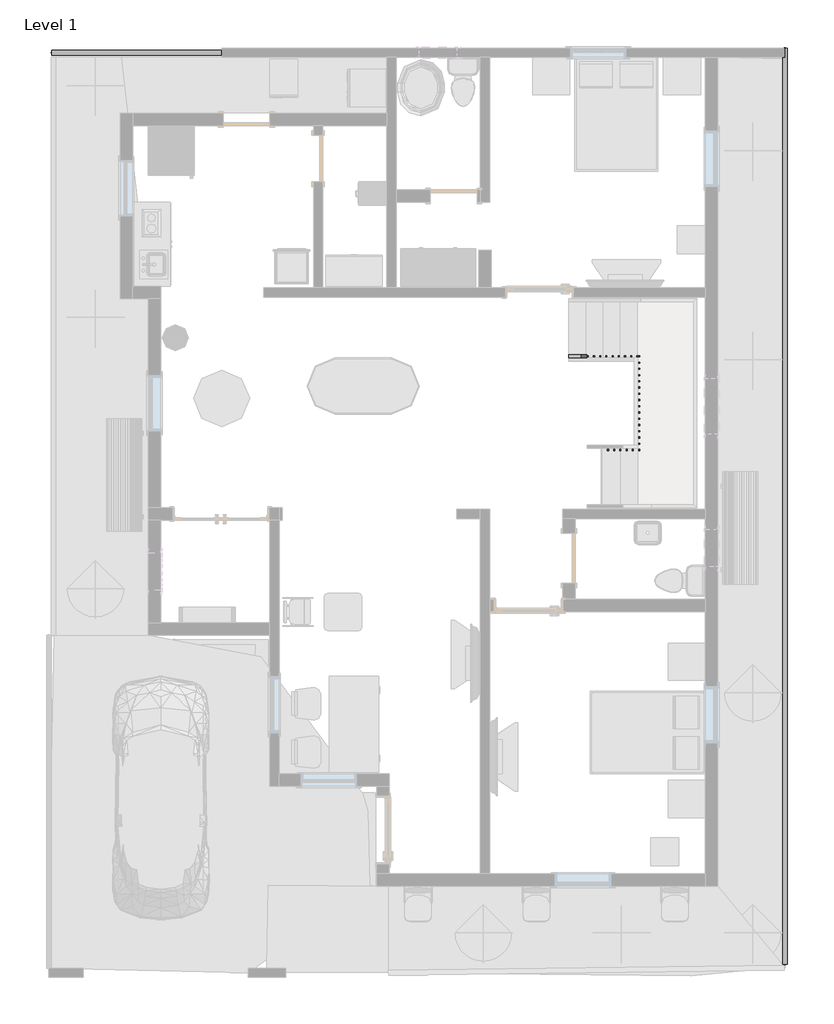
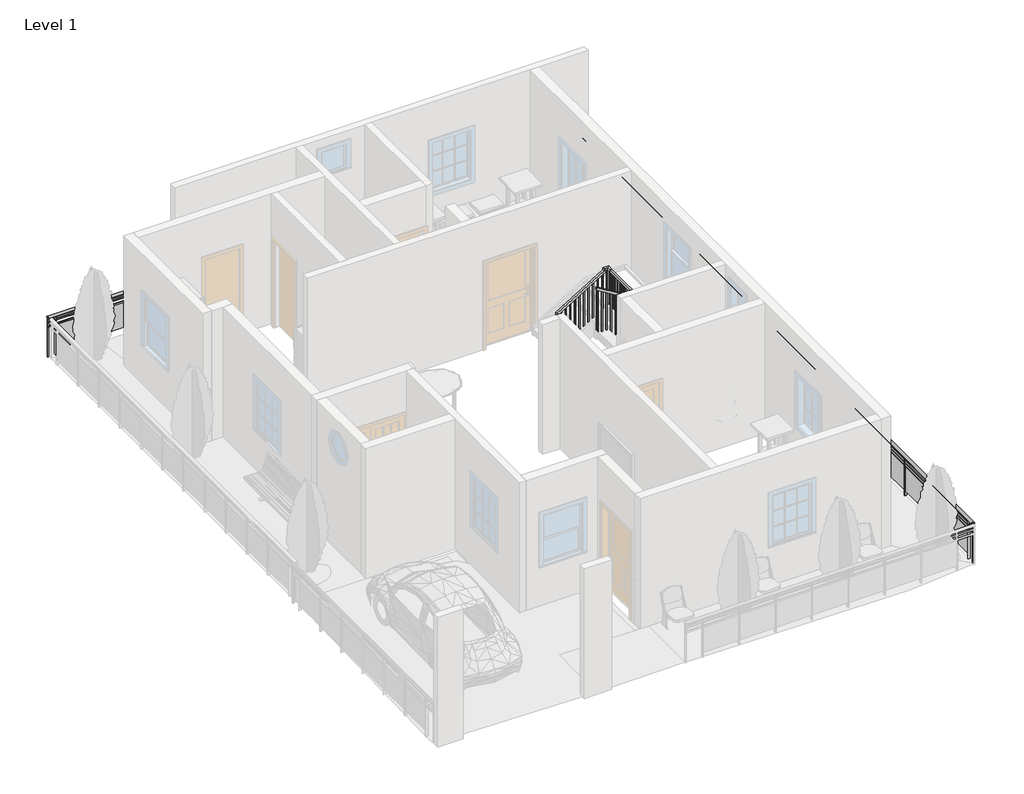
# One storey, part 3 of 4: 3 railings.
"""IFC4 building model written with IfcOpenShell, lengths in millimetres."""

from ifc_helpers import new_model, si_unit, point, frame, origin, origin_with_axes, place, context, project, spatial, polyline, ellipse_curve, trimmed, outline, extrude, faceted_brep, element, save
from ifc_brep_helpers import plane_surface, extruded_surface, advanced_brep

model = new_model("IFC4")

# Units and contexts
model_context = context("Model", 3, world=origin())
ifc_project = project(units=[si_unit("LENGTHUNIT", "METRE", prefix="MILLI")], contexts=[model_context])

# Site, building, storey
site = spatial("IfcSite", under=ifc_project)
building = spatial("IfcBuilding", under=site)
storey = spatial("IfcBuildingStorey", under=building, Name="Level 1", Elevation=0.0)

# Railings
placement = place(None, origin())
element("IfcRailing", 1, ObjectType="Glass Panel - Bottom Fill", at=placement, inside=storey, context=model_context, shape_type="SolidModel", body=[
    advanced_brep(
    [(-5161.8434793, 15525.6426639, 914.4), (-5238.0434793, 15525.6426639, 914.4), (-5161.8434793, 590.4426639, 914.4), (-5238.0434793, 590.4426639, 914.4)],
    [
        (0, 1, ellipse_curve(frame((-5199.9434793, 15525.6426639, 914.4), z_axis=(0.0, 1.0, 0.0), x_axis=(-1.0, 0.0, 0.0)), 38.1, 28.575)),
        (1, 0, ellipse_curve(frame((-5199.9434793, 15525.6426639, 914.4), z_axis=(0.0, 1.0, 0.0), x_axis=(-1.0, 0.0, 0.0)), 38.1, 28.575)),
        (2, 3, ellipse_curve(frame((-5199.9434793, 590.4426639, 914.4), z_axis=(0.0, -1.0, 0.0), x_axis=(-1.0, 0.0, 0.0)), 38.1, 28.575)),
        (3, 2, ellipse_curve(frame((-5199.9434793, 590.4426639, 914.4), z_axis=(0.0, -1.0, 0.0), x_axis=(-1.0, 0.0, 0.0)), 38.1, 28.575)),
        (0, 2),
        (3, 1),
    ],
    [
        plane_surface(frame((-5199.9434793, 15525.6426639, 914.4), z_axis=(0.0, 1.0, 0.0), x_axis=(0.0, 0.0, -1.0))),
        plane_surface(frame((-5199.9434793, 590.4426639, 914.4), z_axis=(0.0, -1.0, 0.0), x_axis=(0.0, 0.0, -1.0))),
        extruded_surface(trimmed(ellipse_curve(frame((-5199.9434793, 590.4426639, 914.4), z_axis=(0.0, 1.0, 0.0), x_axis=(-1.0, 0.0, 0.0)), 38.1, 28.575), [point((-5161.8434793, 590.4426639, 914.4))], [point((-5238.0434793, 590.4426639, 914.4))], True, "CARTESIAN"), (0.0, 14935.2, 0.0), 14935.2),
        extruded_surface(trimmed(ellipse_curve(frame((-5199.9434793, 590.4426639, 914.4), z_axis=(0.0, 1.0, 0.0), x_axis=(-1.0, 0.0, 0.0)), 38.1, 28.575), [point((-5238.0434793, 590.4426639, 914.4))], [point((-5161.8434793, 590.4426639, 914.4))], True, "CARTESIAN"), (0.0, 14935.2, 0.0), 14935.2),
    ],
    [
        (0, [[1, 2]]),
        (1, [[3, 4]]),
        (2, [[-1, 5, -4, 6]]),
        (3, [[-2, -6, -3, -5]]),
    ],
),
    extrude(outline(polyline([(-5212.6434793, 15525.6426639), (-5187.2434793, 15525.6426639), (-5187.2434793, 590.4426639), (-5212.6434793, 590.4426639), (-5212.6434793, 15525.6426639)])), frame((0.0, 0.0, 800.1), z_axis=(0.0, 0.0, 1.0), x_axis=(1.0, 0.0, 0.0)), (0.0, 0.0, 1.0), 25.4),
    extrude(outline(polyline([(-5212.6434793, 15525.6426639), (-5187.2434793, 15525.6426639), (-5187.2434793, 590.4426639), (-5212.6434793, 590.4426639), (-5212.6434793, 15525.6426639)])), frame((0.0, 0.0, 698.5), z_axis=(0.0, 0.0, 1.0), x_axis=(1.0, 0.0, 0.0)), (0.0, 0.0, 1.0), 25.4),
    extrude(outline(polyline([(-5225.3434793, 749.1926639), (-5174.5434793, 749.1926639), (-5174.5434793, 736.4926639), (-5225.3434793, 736.4926639), (-5225.3434793, 749.1926639)])), origin_with_axes(), (0.0, 0.0, 1.0), 885.6788223),
    extrude(outline(polyline([(-5193.4083223, 1555.6426639), (-5193.4083223, 742.8426639), (-5199.7583223, 742.8426639), (-5199.7583223, 1555.6426639), (-5193.4083223, 1555.6426639)])), frame((0.0, 0.0, 101.6), z_axis=(0.0, 0.0, 1.0), x_axis=(1.0, 0.0, 0.0)), (0.0, 0.0, 1.0), 596.9),
    extrude(outline(polyline([(-5225.3434793, 1561.9926639), (-5174.5434793, 1561.9926639), (-5174.5434793, 1549.2926639), (-5225.3434793, 1549.2926639), (-5225.3434793, 1561.9926639)])), origin_with_axes(), (0.0, 0.0, 1.0), 885.6788223),
    extrude(outline(polyline([(-5193.4083223, 2368.4426639), (-5193.4083223, 1555.6426639), (-5199.7583223, 1555.6426639), (-5199.7583223, 2368.4426639), (-5193.4083223, 2368.4426639)])), frame((0.0, 0.0, 101.6), z_axis=(0.0, 0.0, 1.0), x_axis=(1.0, 0.0, 0.0)), (0.0, 0.0, 1.0), 596.9),
    extrude(outline(polyline([(-5225.3434793, 2374.7926639), (-5174.5434793, 2374.7926639), (-5174.5434793, 2362.0926639), (-5225.3434793, 2362.0926639), (-5225.3434793, 2374.7926639)])), origin_with_axes(), (0.0, 0.0, 1.0), 885.6788223),
    extrude(outline(polyline([(-5193.4083223, 3181.2426639), (-5193.4083223, 2368.4426639), (-5199.7583223, 2368.4426639), (-5199.7583223, 3181.2426639), (-5193.4083223, 3181.2426639)])), frame((0.0, 0.0, 101.6), z_axis=(0.0, 0.0, 1.0), x_axis=(1.0, 0.0, 0.0)), (0.0, 0.0, 1.0), 596.9),
    extrude(outline(polyline([(-5225.3434793, 3187.5926639), (-5174.5434793, 3187.5926639), (-5174.5434793, 3174.8926639), (-5225.3434793, 3174.8926639), (-5225.3434793, 3187.5926639)])), origin_with_axes(), (0.0, 0.0, 1.0), 885.6788223),
    extrude(outline(polyline([(-5193.4083223, 3994.0426639), (-5193.4083223, 3181.2426639), (-5199.7583223, 3181.2426639), (-5199.7583223, 3994.0426639), (-5193.4083223, 3994.0426639)])), frame((0.0, 0.0, 101.6), z_axis=(0.0, 0.0, 1.0), x_axis=(1.0, 0.0, 0.0)), (0.0, 0.0, 1.0), 596.9),
    extrude(outline(polyline([(-5225.3434793, 4000.3926639), (-5174.5434793, 4000.3926639), (-5174.5434793, 3987.6926639), (-5225.3434793, 3987.6926639), (-5225.3434793, 4000.3926639)])), origin_with_axes(), (0.0, 0.0, 1.0), 885.6788223),
    extrude(outline(polyline([(-5193.4083223, 4806.8426639), (-5193.4083223, 3994.0426639), (-5199.7583223, 3994.0426639), (-5199.7583223, 4806.8426639), (-5193.4083223, 4806.8426639)])), frame((0.0, 0.0, 101.6), z_axis=(0.0, 0.0, 1.0), x_axis=(1.0, 0.0, 0.0)), (0.0, 0.0, 1.0), 596.9),
    extrude(outline(polyline([(-5225.3434793, 4813.1926639), (-5174.5434793, 4813.1926639), (-5174.5434793, 4800.4926639), (-5225.3434793, 4800.4926639), (-5225.3434793, 4813.1926639)])), origin_with_axes(), (0.0, 0.0, 1.0), 885.6788223),
    extrude(outline(polyline([(-5193.4083223, 5619.6426639), (-5193.4083223, 4806.8426639), (-5199.7583223, 4806.8426639), (-5199.7583223, 5619.6426639), (-5193.4083223, 5619.6426639)])), frame((0.0, 0.0, 101.6), z_axis=(0.0, 0.0, 1.0), x_axis=(1.0, 0.0, 0.0)), (0.0, 0.0, 1.0), 596.9),
    extrude(outline(polyline([(-5225.3434793, 5625.9926639), (-5174.5434793, 5625.9926639), (-5174.5434793, 5613.2926639), (-5225.3434793, 5613.2926639), (-5225.3434793, 5625.9926639)])), origin_with_axes(), (0.0, 0.0, 1.0), 885.6788223),
    extrude(outline(polyline([(-5193.4083223, 6432.4426639), (-5193.4083223, 5619.6426639), (-5199.7583223, 5619.6426639), (-5199.7583223, 6432.4426639), (-5193.4083223, 6432.4426639)])), frame((0.0, 0.0, 101.6), z_axis=(0.0, 0.0, 1.0), x_axis=(1.0, 0.0, 0.0)), (0.0, 0.0, 1.0), 596.9),
    extrude(outline(polyline([(-5225.3434793, 6438.7926639), (-5174.5434793, 6438.7926639), (-5174.5434793, 6426.0926639), (-5225.3434793, 6426.0926639), (-5225.3434793, 6438.7926639)])), origin_with_axes(), (0.0, 0.0, 1.0), 885.6788223),
    extrude(outline(polyline([(-5193.4083223, 7245.2426639), (-5193.4083223, 6432.4426639), (-5199.7583223, 6432.4426639), (-5199.7583223, 7245.2426639), (-5193.4083223, 7245.2426639)])), frame((0.0, 0.0, 101.6), z_axis=(0.0, 0.0, 1.0), x_axis=(1.0, 0.0, 0.0)), (0.0, 0.0, 1.0), 596.9),
    extrude(outline(polyline([(-5225.3434793, 7251.5926639), (-5174.5434793, 7251.5926639), (-5174.5434793, 7238.8926639), (-5225.3434793, 7238.8926639), (-5225.3434793, 7251.5926639)])), origin_with_axes(), (0.0, 0.0, 1.0), 885.6788223),
    extrude(outline(polyline([(-5193.4083223, 8058.0426639), (-5193.4083223, 7245.2426639), (-5199.7583223, 7245.2426639), (-5199.7583223, 8058.0426639), (-5193.4083223, 8058.0426639)])), frame((0.0, 0.0, 101.6), z_axis=(0.0, 0.0, 1.0), x_axis=(1.0, 0.0, 0.0)), (0.0, 0.0, 1.0), 596.9),
    extrude(outline(polyline([(-5225.3434793, 8064.3926639), (-5174.5434793, 8064.3926639), (-5174.5434793, 8051.6926639), (-5225.3434793, 8051.6926639), (-5225.3434793, 8064.3926639)])), origin_with_axes(), (0.0, 0.0, 1.0), 885.6788223),
    extrude(outline(polyline([(-5193.4083223, 8870.8426639), (-5193.4083223, 8058.0426639), (-5199.7583223, 8058.0426639), (-5199.7583223, 8870.8426639), (-5193.4083223, 8870.8426639)])), frame((0.0, 0.0, 101.6), z_axis=(0.0, 0.0, 1.0), x_axis=(1.0, 0.0, 0.0)), (0.0, 0.0, 1.0), 596.9),
    extrude(outline(polyline([(-5225.3434793, 8877.1926639), (-5174.5434793, 8877.1926639), (-5174.5434793, 8864.4926639), (-5225.3434793, 8864.4926639), (-5225.3434793, 8877.1926639)])), origin_with_axes(), (0.0, 0.0, 1.0), 885.6788223),
    extrude(outline(polyline([(-5193.4083223, 9683.6426639), (-5193.4083223, 8870.8426639), (-5199.7583223, 8870.8426639), (-5199.7583223, 9683.6426639), (-5193.4083223, 9683.6426639)])), frame((0.0, 0.0, 101.6), z_axis=(0.0, 0.0, 1.0), x_axis=(1.0, 0.0, 0.0)), (0.0, 0.0, 1.0), 596.9),
    extrude(outline(polyline([(-5225.3434793, 9689.9926639), (-5174.5434793, 9689.9926639), (-5174.5434793, 9677.2926639), (-5225.3434793, 9677.2926639), (-5225.3434793, 9689.9926639)])), origin_with_axes(), (0.0, 0.0, 1.0), 885.6788223),
    extrude(outline(polyline([(-5193.4083223, 10496.4426639), (-5193.4083223, 9683.6426639), (-5199.7583223, 9683.6426639), (-5199.7583223, 10496.4426639), (-5193.4083223, 10496.4426639)])), frame((0.0, 0.0, 101.6), z_axis=(0.0, 0.0, 1.0), x_axis=(1.0, 0.0, 0.0)), (0.0, 0.0, 1.0), 596.9),
    extrude(outline(polyline([(-5225.3434793, 10502.7926639), (-5174.5434793, 10502.7926639), (-5174.5434793, 10490.0926639), (-5225.3434793, 10490.0926639), (-5225.3434793, 10502.7926639)])), origin_with_axes(), (0.0, 0.0, 1.0), 885.6788223),
    extrude(outline(polyline([(-5193.4083223, 11309.2426639), (-5193.4083223, 10496.4426639), (-5199.7583223, 10496.4426639), (-5199.7583223, 11309.2426639), (-5193.4083223, 11309.2426639)])), frame((0.0, 0.0, 101.6), z_axis=(0.0, 0.0, 1.0), x_axis=(1.0, 0.0, 0.0)), (0.0, 0.0, 1.0), 596.9),
    extrude(outline(polyline([(-5225.3434793, 11315.5926639), (-5174.5434793, 11315.5926639), (-5174.5434793, 11302.8926639), (-5225.3434793, 11302.8926639), (-5225.3434793, 11315.5926639)])), origin_with_axes(), (0.0, 0.0, 1.0), 885.6788223),
    extrude(outline(polyline([(-5193.4083223, 12122.0426639), (-5193.4083223, 11309.2426639), (-5199.7583223, 11309.2426639), (-5199.7583223, 12122.0426639), (-5193.4083223, 12122.0426639)])), frame((0.0, 0.0, 101.6), z_axis=(0.0, 0.0, 1.0), x_axis=(1.0, 0.0, 0.0)), (0.0, 0.0, 1.0), 596.9),
    extrude(outline(polyline([(-5225.3434793, 12128.3926639), (-5174.5434793, 12128.3926639), (-5174.5434793, 12115.6926639), (-5225.3434793, 12115.6926639), (-5225.3434793, 12128.3926639)])), origin_with_axes(), (0.0, 0.0, 1.0), 885.6788223),
    extrude(outline(polyline([(-5193.4083223, 12934.8426639), (-5193.4083223, 12122.0426639), (-5199.7583223, 12122.0426639), (-5199.7583223, 12934.8426639), (-5193.4083223, 12934.8426639)])), frame((0.0, 0.0, 101.6), z_axis=(0.0, 0.0, 1.0), x_axis=(1.0, 0.0, 0.0)), (0.0, 0.0, 1.0), 596.9),
    extrude(outline(polyline([(-5225.3434793, 12941.1926639), (-5174.5434793, 12941.1926639), (-5174.5434793, 12928.4926639), (-5225.3434793, 12928.4926639), (-5225.3434793, 12941.1926639)])), origin_with_axes(), (0.0, 0.0, 1.0), 885.6788223),
    extrude(outline(polyline([(-5193.4083223, 13747.6426639), (-5193.4083223, 12934.8426639), (-5199.7583223, 12934.8426639), (-5199.7583223, 13747.6426639), (-5193.4083223, 13747.6426639)])), frame((0.0, 0.0, 101.6), z_axis=(0.0, 0.0, 1.0), x_axis=(1.0, 0.0, 0.0)), (0.0, 0.0, 1.0), 596.9),
    extrude(outline(polyline([(-5225.3434793, 13753.9926639), (-5174.5434793, 13753.9926639), (-5174.5434793, 13741.2926639), (-5225.3434793, 13741.2926639), (-5225.3434793, 13753.9926639)])), origin_with_axes(), (0.0, 0.0, 1.0), 885.6788223),
    extrude(outline(polyline([(-5193.4083223, 14560.4426639), (-5193.4083223, 13747.6426639), (-5199.7583223, 13747.6426639), (-5199.7583223, 14560.4426639), (-5193.4083223, 14560.4426639)])), frame((0.0, 0.0, 101.6), z_axis=(0.0, 0.0, 1.0), x_axis=(1.0, 0.0, 0.0)), (0.0, 0.0, 1.0), 596.9),
    extrude(outline(polyline([(-5225.3434793, 14566.7926639), (-5174.5434793, 14566.7926639), (-5174.5434793, 14554.0926639), (-5225.3434793, 14554.0926639), (-5225.3434793, 14566.7926639)])), origin_with_axes(), (0.0, 0.0, 1.0), 885.6788223),
    extrude(outline(polyline([(-5193.4083223, 15373.2426639), (-5193.4083223, 14560.4426639), (-5199.7583223, 14560.4426639), (-5199.7583223, 15373.2426639), (-5193.4083223, 15373.2426639)])), frame((0.0, 0.0, 101.6), z_axis=(0.0, 0.0, 1.0), x_axis=(1.0, 0.0, 0.0)), (0.0, 0.0, 1.0), 596.9),
    extrude(outline(polyline([(-5225.3434793, 15379.5926639), (-5174.5434793, 15379.5926639), (-5174.5434793, 15366.8926639), (-5225.3434793, 15366.8926639), (-5225.3434793, 15379.5926639)])), origin_with_axes(), (0.0, 0.0, 1.0), 885.6788223),
    extrude(outline(polyline([(-5209.4684793, 603.1426639), (-5190.4184793, 603.1426639), (-5190.4184793, 584.0926639), (-5209.4684793, 584.0926639), (-5209.4684793, 603.1426639)])), origin_with_axes(), (0.0, 0.0, 1.0), 885.6788223),
    extrude(outline(polyline([(-5209.4684793, 15531.9926639), (-5190.4184793, 15531.9926639), (-5190.4184793, 15512.9426639), (-5209.4684793, 15512.9426639), (-5209.4684793, 15531.9926639)])), origin_with_axes(), (0.0, 0.0, 1.0), 885.6788223),
])
element("IfcRailing", 2, ObjectType="Glass Panel - Bottom Fill", at=placement, inside=storey, context=model_context, shape_type="SolidModel", body=[
    advanced_brep(
    [(-17152.6399968, 15487.5426639, 914.4), (-17152.6399968, 15411.3426639, 914.4), (-14384.0399968, 15487.5426639, 914.4), (-14384.0399968, 15411.3426639, 914.4)],
    [
        (0, 1, ellipse_curve(frame((-17152.6399968, 15449.4426639, 914.4), z_axis=(-1.0, 0.0, 0.0), x_axis=(0.0, -1.0, 0.0)), 38.1, 28.575)),
        (1, 0, ellipse_curve(frame((-17152.6399968, 15449.4426639, 914.4), z_axis=(-1.0, 0.0, 0.0), x_axis=(0.0, -1.0, 0.0)), 38.1, 28.575)),
        (2, 3, ellipse_curve(frame((-14384.0399968, 15449.4426639, 914.4), z_axis=(1.0, 0.0, 0.0), x_axis=(0.0, -1.0, 0.0)), 38.1, 28.575)),
        (3, 2, ellipse_curve(frame((-14384.0399968, 15449.4426639, 914.4), z_axis=(1.0, 0.0, 0.0), x_axis=(0.0, -1.0, 0.0)), 38.1, 28.575)),
        (0, 2),
        (3, 1),
    ],
    [
        plane_surface(frame((-17152.6399968, 15449.4426639, 914.4), z_axis=(-1.0, 0.0, 0.0), x_axis=(0.0, 1.0, 0.0))),
        plane_surface(frame((-14384.0399968, 15449.4426639, 914.4), z_axis=(1.0, 0.0, 0.0), x_axis=(0.0, 1.0, 0.0))),
        extruded_surface(trimmed(ellipse_curve(frame((-14384.0399968, 15449.4426639, 914.4), z_axis=(-1.0, 0.0, 0.0), x_axis=(0.0, -1.0, 0.0)), 38.1, 28.575), [point((-14384.0399968, 15487.5426639, 914.4))], [point((-14384.0399968, 15411.3426639, 914.4))], True, "CARTESIAN"), (-2768.6000000000004, 0.0, 0.0), 2768.6000000000004),
        extruded_surface(trimmed(ellipse_curve(frame((-14384.0399968, 15449.4426639, 914.4), z_axis=(-1.0, 0.0, 0.0), x_axis=(0.0, -1.0, 0.0)), 38.1, 28.575), [point((-14384.0399968, 15411.3426639, 914.4))], [point((-14384.0399968, 15487.5426639, 914.4))], True, "CARTESIAN"), (-2768.6000000000004, 0.0, 0.0), 2768.6000000000004),
    ],
    [
        (0, [[1, 2]]),
        (1, [[3, 4]]),
        (2, [[-1, 5, -4, 6]]),
        (3, [[-2, -6, -3, -5]]),
    ],
),
    extrude(outline(polyline([(-17152.6399968, 15436.7426639), (-17152.6399968, 15462.1426639), (-14384.0399968, 15462.1426639), (-14384.0399968, 15436.7426639), (-17152.6399968, 15436.7426639)])), frame((0.0, 0.0, 800.1), z_axis=(0.0, 0.0, 1.0), x_axis=(1.0, 0.0, 0.0)), (0.0, 0.0, 1.0), 25.4),
    extrude(outline(polyline([(-17152.6399968, 15436.7426639), (-17152.6399968, 15462.1426639), (-14384.0399968, 15462.1426639), (-14384.0399968, 15436.7426639), (-17152.6399968, 15436.7426639)])), frame((0.0, 0.0, 698.5), z_axis=(0.0, 0.0, 1.0), x_axis=(1.0, 0.0, 0.0)), (0.0, 0.0, 1.0), 25.4),
    extrude(outline(polyline([(-14555.4899968, 15424.0426639), (-14555.4899968, 15474.8426639), (-14542.7899968, 15474.8426639), (-14542.7899968, 15424.0426639), (-14555.4899968, 15424.0426639)])), origin_with_axes(), (0.0, 0.0, 1.0), 885.6788223),
    extrude(outline(polyline([(-15361.9399968, 15455.9778209), (-14549.1399968, 15455.9778209), (-14549.1399968, 15449.6278209), (-15361.9399968, 15449.6278209), (-15361.9399968, 15455.9778209)])), frame((0.0, 0.0, 101.6), z_axis=(0.0, 0.0, 1.0), x_axis=(1.0, 0.0, 0.0)), (0.0, 0.0, 1.0), 596.9),
    extrude(outline(polyline([(-15368.2899968, 15424.0426639), (-15368.2899968, 15474.8426639), (-15355.5899968, 15474.8426639), (-15355.5899968, 15424.0426639), (-15368.2899968, 15424.0426639)])), origin_with_axes(), (0.0, 0.0, 1.0), 885.6788223),
    extrude(outline(polyline([(-16174.7399968, 15455.9778209), (-15361.9399968, 15455.9778209), (-15361.9399968, 15449.6278209), (-16174.7399968, 15449.6278209), (-16174.7399968, 15455.9778209)])), frame((0.0, 0.0, 101.6), z_axis=(0.0, 0.0, 1.0), x_axis=(1.0, 0.0, 0.0)), (0.0, 0.0, 1.0), 596.9),
    extrude(outline(polyline([(-16181.0899968, 15424.0426639), (-16181.0899968, 15474.8426639), (-16168.3899968, 15474.8426639), (-16168.3899968, 15424.0426639), (-16181.0899968, 15424.0426639)])), origin_with_axes(), (0.0, 0.0, 1.0), 885.6788223),
    extrude(outline(polyline([(-16987.5399968, 15455.9778209), (-16174.7399968, 15455.9778209), (-16174.7399968, 15449.6278209), (-16987.5399968, 15449.6278209), (-16987.5399968, 15455.9778209)])), frame((0.0, 0.0, 101.6), z_axis=(0.0, 0.0, 1.0), x_axis=(1.0, 0.0, 0.0)), (0.0, 0.0, 1.0), 596.9),
    extrude(outline(polyline([(-16993.8899968, 15424.0426639), (-16993.8899968, 15474.8426639), (-16981.1899968, 15474.8426639), (-16981.1899968, 15424.0426639), (-16993.8899968, 15424.0426639)])), origin_with_axes(), (0.0, 0.0, 1.0), 885.6788223),
    extrude(outline(polyline([(-14396.7399968, 15439.9176639), (-14396.7399968, 15458.9676639), (-14377.6899968, 15458.9676639), (-14377.6899968, 15439.9176639), (-14396.7399968, 15439.9176639)])), origin_with_axes(), (0.0, 0.0, 1.0), 885.6788223),
    extrude(outline(polyline([(-17158.9899968, 15439.9176639), (-17158.9899968, 15458.9676639), (-17139.9399968, 15458.9676639), (-17139.9399968, 15439.9176639), (-17158.9899968, 15439.9176639)])), origin_with_axes(), (0.0, 0.0, 1.0), 885.6788223),
])
element("IfcRailing", 3, ObjectType="Handrail - Rectangular", at=placement, inside=storey, context=model_context, shape_type="SolidModel", body=[
    faceted_brep([(-8719.8399968, 10524.1610583, 1083.7333333), (-8719.8399968, 10524.1610583, 1024.3318731), (-8719.8399968, 10473.3610583, 1024.3318731), (-8719.8399968, 10473.3610583, 1083.7333333), (-7678.4399968, 10524.1610583, 1714.8848485), (-7627.6399968, 10524.1610583, 1686.271267), (-7627.6399968, 10473.3610583, 1686.271267), (-7678.4399968, 10473.3610583, 1714.8848485), (-7678.4399968, 10524.1610583, 1761.0666667), (-7627.6399968, 10524.1610583, 1710.2666667), (-7627.6399968, 10473.3610583, 1710.2666667), (-7678.4399968, 10473.3610583, 1761.0666667), (-7551.4399968, 10524.1610583, 1761.0666667), (-7551.4399968, 10524.1610583, 1710.2666667), (-7602.2399968, 10473.3610583, 1710.2666667), (-7602.2399968, 10473.3610583, 1761.0666667), (-7551.4399968, 10397.1610583, 1761.0666667), (-7551.4399968, 10397.1610583, 1710.2666667), (-7602.2399968, 10397.1610583, 1710.2666667), (-7602.2399968, 10397.1610583, 1761.0666667), (-7551.4399968, 9074.0426639, 1761.0666667), (-7551.4399968, 9023.2426639, 1710.2666667), (-7602.2399968, 9023.2426639, 1710.2666667), (-7602.2399968, 9074.0426639, 1761.0666667), (-7551.4399968, 9074.0426639, 1976.5818182), (-7551.4399968, 9023.2426639, 1925.7818182), (-7602.2399968, 9023.2426639, 1925.7818182), (-7602.2399968, 9074.0426639, 1976.5818182), (-7551.4399968, 8947.0426639, 1976.5818182), (-7551.4399968, 8947.0426639, 1925.7818182), (-7602.2399968, 8997.8426639, 1925.7818182), (-7602.2399968, 8997.8426639, 1976.5818182), (-7678.4399968, 8947.0426639, 1976.5818182), (-7692.6324062, 8947.0426639, 1925.7818182), (-7692.6324062, 8997.8426639, 1925.7818182), (-7678.4399968, 8997.8426639, 1976.5818182), (-8719.8399968, 8947.0426639, 2607.7333333), (-8719.8399968, 8997.8426639, 2607.7333333), (-8719.8399968, 8997.8426639, 2548.3318731), (-8719.8399968, 8947.0426639, 2548.3318731)], [[[0, 1, 2, 3]], [[1, 0, 4, 5]], [[2, 1, 5, 6]], [[3, 2, 6, 7]], [[0, 3, 7, 4]], [[5, 4, 8, 9]], [[6, 5, 9, 10]], [[7, 6, 10, 11]], [[4, 7, 11, 8]], [[9, 8, 12, 13]], [[10, 9, 13, 14]], [[11, 10, 14, 15]], [[8, 11, 15, 12]], [[13, 12, 16, 17]], [[14, 13, 17, 18]], [[15, 14, 18, 19]], [[12, 15, 19, 16]], [[17, 16, 20, 21]], [[18, 17, 21, 22]], [[19, 18, 22, 23]], [[16, 19, 23, 20]], [[21, 20, 24, 25]], [[22, 21, 25, 26]], [[23, 22, 26, 27]], [[20, 23, 27, 24]], [[25, 24, 28, 29]], [[26, 25, 29, 30]], [[27, 26, 30, 31]], [[24, 27, 31, 28]], [[29, 28, 32, 33]], [[30, 29, 33, 34]], [[31, 30, 34, 35]], [[28, 31, 35, 32]], [[36, 37, 38, 39]], [[33, 32, 36, 39]], [[34, 33, 39, 38]], [[35, 34, 38, 37]], [[32, 35, 37, 36]]]),
    extrude(outline(polyline([(2527.1652064, -8684.9149968), (2538.710661, -8703.9649968), (1524.0, -8703.9649968), (1524.0, -8684.9149968), (2527.1652064, -8684.9149968)])), frame((0.0, 8962.9176639, 0.0), z_axis=(0.0, 1.0, 0.0), x_axis=(0.0, 0.0, 1.0)), (0.0, 0.0, 1.0), 19.05),
    extrude(outline(polyline([(2465.5894488, -8583.3149968), (2477.1349034, -8602.3649968), (1524.0, -8602.3649968), (1524.0, -8583.3149968), (2465.5894488, -8583.3149968)])), frame((0.0, 8962.9176639, 0.0), z_axis=(0.0, 1.0, 0.0), x_axis=(0.0, 0.0, 1.0)), (0.0, 0.0, 1.0), 19.05),
    extrude(outline(polyline([(2404.0136913, -8481.7149968), (2415.5591458, -8500.7649968), (1524.0, -8500.7649968), (1524.0, -8481.7149968), (2404.0136913, -8481.7149968)])), frame((0.0, 8962.9176639, 0.0), z_axis=(0.0, 1.0, 0.0), x_axis=(0.0, 0.0, 1.0)), (0.0, 0.0, 1.0), 19.05),
    extrude(outline(polyline([(2342.4379337, -8380.1149968), (2353.9833882, -8399.1649968), (1354.6666667, -8399.1649968), (1354.6666667, -8380.1149968), (2342.4379337, -8380.1149968)])), frame((0.0, 8962.9176639, 0.0), z_axis=(0.0, 1.0, 0.0), x_axis=(0.0, 0.0, 1.0)), (0.0, 0.0, 1.0), 19.05),
    extrude(outline(polyline([(2280.8621761, -8278.5149968), (2292.4076307, -8297.5649968), (1354.6666667, -8297.5649968), (1354.6666667, -8278.5149968), (2280.8621761, -8278.5149968)])), frame((0.0, 8962.9176639, 0.0), z_axis=(0.0, 1.0, 0.0), x_axis=(0.0, 0.0, 1.0)), (0.0, 0.0, 1.0), 19.05),
    extrude(outline(polyline([(2219.2864185, -8176.9149968), (2230.8318731, -8195.9649968), (1354.6666667, -8195.9649968), (1354.6666667, -8176.9149968), (2219.2864185, -8176.9149968)])), frame((0.0, 8962.9176639, 0.0), z_axis=(0.0, 1.0, 0.0), x_axis=(0.0, 0.0, 1.0)), (0.0, 0.0, 1.0), 19.05),
    extrude(outline(polyline([(2157.710661, -8075.3149968), (2169.2561155, -8094.3649968), (1185.3333333, -8094.3649968), (1185.3333333, -8075.3149968), (2157.710661, -8075.3149968)])), frame((0.0, 8962.9176639, 0.0), z_axis=(0.0, 1.0, 0.0), x_axis=(0.0, 0.0, 1.0)), (0.0, 0.0, 1.0), 19.05),
    extrude(outline(polyline([(2096.1349034, -7973.7149968), (2107.6803579, -7992.7649968), (1185.3333333, -7992.7649968), (1185.3333333, -7973.7149968), (2096.1349034, -7973.7149968)])), frame((0.0, 8962.9176639, 0.0), z_axis=(0.0, 1.0, 0.0), x_axis=(0.0, 0.0, 1.0)), (0.0, 0.0, 1.0), 19.05),
    extrude(outline(polyline([(2034.5591458, -7872.1149968), (2046.1046004, -7891.1649968), (1185.3333333, -7891.1649968), (1185.3333333, -7872.1149968), (2034.5591458, -7872.1149968)])), frame((0.0, 8962.9176639, 0.0), z_axis=(0.0, 1.0, 0.0), x_axis=(0.0, 0.0, 1.0)), (0.0, 0.0, 1.0), 19.05),
    extrude(outline(polyline([(1972.9833882, -7770.5149968), (1984.5288428, -7789.5649968), (1016.0, -7789.5649968), (1016.0, -7770.5149968), (1972.9833882, -7770.5149968)])), frame((0.0, 8962.9176639, 0.0), z_axis=(0.0, 1.0, 0.0), x_axis=(0.0, 0.0, 1.0)), (0.0, 0.0, 1.0), 19.05),
    extrude(outline(polyline([(-7668.9149968, 8981.9676639), (-7668.9149968, 8962.9176639), (-7687.9649968, 8962.9176639), (-7687.9649968, 8981.9676639), (-7668.9149968, 8981.9676639)])), frame((0.0, 0.0, 1016.0), z_axis=(0.0, 0.0, 1.0), x_axis=(1.0, 0.0, 0.0)), (0.0, 0.0, 1.0), 909.7818182),
    extrude(outline(polyline([(-7586.3649968, 8984.2860583), (-7567.3149968, 8984.2860583), (-7567.3149968, 8965.2360583), (-7586.3649968, 8965.2360583), (-7586.3649968, 8984.2860583)])), frame((0.0, 0.0, 846.6666667), z_axis=(0.0, 0.0, 1.0), x_axis=(1.0, 0.0, 0.0)), (0.0, 0.0, 1.0), 1079.1151515),
    extrude(outline(polyline([(-7586.3649968, 9085.8860583), (-7567.3149968, 9085.8860583), (-7567.3149968, 9066.8360583), (-7586.3649968, 9066.8360583), (-7586.3649968, 9085.8860583)])), frame((0.0, 0.0, 846.6666667), z_axis=(0.0, 0.0, 1.0), x_axis=(1.0, 0.0, 0.0)), (0.0, 0.0, 1.0), 863.6),
    extrude(outline(polyline([(-7586.3649968, 9187.4860583), (-7567.3149968, 9187.4860583), (-7567.3149968, 9168.4360583), (-7586.3649968, 9168.4360583), (-7586.3649968, 9187.4860583)])), frame((0.0, 0.0, 846.6666667), z_axis=(0.0, 0.0, 1.0), x_axis=(1.0, 0.0, 0.0)), (0.0, 0.0, 1.0), 863.6),
    extrude(outline(polyline([(-7586.3649968, 9289.0860583), (-7567.3149968, 9289.0860583), (-7567.3149968, 9270.0360583), (-7586.3649968, 9270.0360583), (-7586.3649968, 9289.0860583)])), frame((0.0, 0.0, 846.6666667), z_axis=(0.0, 0.0, 1.0), x_axis=(1.0, 0.0, 0.0)), (0.0, 0.0, 1.0), 863.6),
    extrude(outline(polyline([(-7586.3649968, 9390.6860583), (-7567.3149968, 9390.6860583), (-7567.3149968, 9371.6360583), (-7586.3649968, 9371.6360583), (-7586.3649968, 9390.6860583)])), frame((0.0, 0.0, 846.6666667), z_axis=(0.0, 0.0, 1.0), x_axis=(1.0, 0.0, 0.0)), (0.0, 0.0, 1.0), 863.6),
    extrude(outline(polyline([(-7586.3649968, 9492.2860583), (-7567.3149968, 9492.2860583), (-7567.3149968, 9473.2360583), (-7586.3649968, 9473.2360583), (-7586.3649968, 9492.2860583)])), frame((0.0, 0.0, 846.6666667), z_axis=(0.0, 0.0, 1.0), x_axis=(1.0, 0.0, 0.0)), (0.0, 0.0, 1.0), 863.6),
    extrude(outline(polyline([(-7586.3649968, 9593.8860583), (-7567.3149968, 9593.8860583), (-7567.3149968, 9574.8360583), (-7586.3649968, 9574.8360583), (-7586.3649968, 9593.8860583)])), frame((0.0, 0.0, 846.6666667), z_axis=(0.0, 0.0, 1.0), x_axis=(1.0, 0.0, 0.0)), (0.0, 0.0, 1.0), 863.6),
    extrude(outline(polyline([(-7586.3649968, 9695.4860583), (-7567.3149968, 9695.4860583), (-7567.3149968, 9676.4360583), (-7586.3649968, 9676.4360583), (-7586.3649968, 9695.4860583)])), frame((0.0, 0.0, 846.6666667), z_axis=(0.0, 0.0, 1.0), x_axis=(1.0, 0.0, 0.0)), (0.0, 0.0, 1.0), 863.6),
    extrude(outline(polyline([(-7586.3649968, 9797.0860583), (-7567.3149968, 9797.0860583), (-7567.3149968, 9778.0360583), (-7586.3649968, 9778.0360583), (-7586.3649968, 9797.0860583)])), frame((0.0, 0.0, 846.6666667), z_axis=(0.0, 0.0, 1.0), x_axis=(1.0, 0.0, 0.0)), (0.0, 0.0, 1.0), 863.6),
    extrude(outline(polyline([(-7586.3649968, 9898.6860583), (-7567.3149968, 9898.6860583), (-7567.3149968, 9879.6360583), (-7586.3649968, 9879.6360583), (-7586.3649968, 9898.6860583)])), frame((0.0, 0.0, 846.6666667), z_axis=(0.0, 0.0, 1.0), x_axis=(1.0, 0.0, 0.0)), (0.0, 0.0, 1.0), 863.6),
    extrude(outline(polyline([(-7586.3649968, 10000.2860583), (-7567.3149968, 10000.2860583), (-7567.3149968, 9981.2360583), (-7586.3649968, 9981.2360583), (-7586.3649968, 10000.2860583)])), frame((0.0, 0.0, 846.6666667), z_axis=(0.0, 0.0, 1.0), x_axis=(1.0, 0.0, 0.0)), (0.0, 0.0, 1.0), 863.6),
    extrude(outline(polyline([(-7586.3649968, 10101.8860583), (-7567.3149968, 10101.8860583), (-7567.3149968, 10082.8360583), (-7586.3649968, 10082.8360583), (-7586.3649968, 10101.8860583)])), frame((0.0, 0.0, 846.6666667), z_axis=(0.0, 0.0, 1.0), x_axis=(1.0, 0.0, 0.0)), (0.0, 0.0, 1.0), 863.6),
    extrude(outline(polyline([(-7586.3649968, 10203.4860583), (-7567.3149968, 10203.4860583), (-7567.3149968, 10184.4360583), (-7586.3649968, 10184.4360583), (-7586.3649968, 10203.4860583)])), frame((0.0, 0.0, 846.6666667), z_axis=(0.0, 0.0, 1.0), x_axis=(1.0, 0.0, 0.0)), (0.0, 0.0, 1.0), 863.6),
    extrude(outline(polyline([(-7586.3649968, 10305.0860583), (-7567.3149968, 10305.0860583), (-7567.3149968, 10286.0360583), (-7586.3649968, 10286.0360583), (-7586.3649968, 10305.0860583)])), frame((0.0, 0.0, 846.6666667), z_axis=(0.0, 0.0, 1.0), x_axis=(1.0, 0.0, 0.0)), (0.0, 0.0, 1.0), 863.6),
    extrude(outline(polyline([(-7586.3649968, 10406.6860583), (-7567.3149968, 10406.6860583), (-7567.3149968, 10387.6360583), (-7586.3649968, 10387.6360583), (-7586.3649968, 10406.6860583)])), frame((0.0, 0.0, 846.6666667), z_axis=(0.0, 0.0, 1.0), x_axis=(1.0, 0.0, 0.0)), (0.0, 0.0, 1.0), 863.6),
    extrude(outline(polyline([(1645.8621761, -7694.3149968), (1634.3167216, -7713.3649968), (677.3333333, -7713.3649968), (677.3333333, -7694.3149968), (1645.8621761, -7694.3149968)])), frame((0.0, 10489.2360583, 0.0), z_axis=(0.0, 1.0, 0.0), x_axis=(0.0, 0.0, 1.0)), (0.0, 0.0, 1.0), 19.05),
    extrude(outline(polyline([(1584.2864185, -7795.9149968), (1572.740964, -7814.9649968), (677.3333333, -7814.9649968), (677.3333333, -7795.9149968), (1584.2864185, -7795.9149968)])), frame((0.0, 10489.2360583, 0.0), z_axis=(0.0, 1.0, 0.0), x_axis=(0.0, 0.0, 1.0)), (0.0, 0.0, 1.0), 19.05),
    extrude(outline(polyline([(1522.710661, -7897.5149968), (1511.1652064, -7916.5649968), (508.0, -7916.5649968), (508.0, -7897.5149968), (1522.710661, -7897.5149968)])), frame((0.0, 10489.2360583, 0.0), z_axis=(0.0, 1.0, 0.0), x_axis=(0.0, 0.0, 1.0)), (0.0, 0.0, 1.0), 19.05),
    extrude(outline(polyline([(1461.1349034, -7999.1149968), (1449.5894488, -8018.1649968), (508.0, -8018.1649968), (508.0, -7999.1149968), (1461.1349034, -7999.1149968)])), frame((0.0, 10489.2360583, 0.0), z_axis=(0.0, 1.0, 0.0), x_axis=(0.0, 0.0, 1.0)), (0.0, 0.0, 1.0), 19.05),
    extrude(outline(polyline([(1399.5591458, -8100.7149968), (1388.0136913, -8119.7649968), (508.0, -8119.7649968), (508.0, -8100.7149968), (1399.5591458, -8100.7149968)])), frame((0.0, 10489.2360583, 0.0), z_axis=(0.0, 1.0, 0.0), x_axis=(0.0, 0.0, 1.0)), (0.0, 0.0, 1.0), 19.05),
    extrude(outline(polyline([(1337.9833882, -8202.3149968), (1326.4379337, -8221.3649968), (338.6666667, -8221.3649968), (338.6666667, -8202.3149968), (1337.9833882, -8202.3149968)])), frame((0.0, 10489.2360583, 0.0), z_axis=(0.0, 1.0, 0.0), x_axis=(0.0, 0.0, 1.0)), (0.0, 0.0, 1.0), 19.05),
    extrude(outline(polyline([(1276.4076307, -8303.9149968), (1264.8621761, -8322.9649968), (338.6666667, -8322.9649968), (338.6666667, -8303.9149968), (1276.4076307, -8303.9149968)])), frame((0.0, 10489.2360583, 0.0), z_axis=(0.0, 1.0, 0.0), x_axis=(0.0, 0.0, 1.0)), (0.0, 0.0, 1.0), 19.05),
    extrude(outline(polyline([(1214.8318731, -8405.5149968), (1203.2864185, -8424.5649968), (338.6666667, -8424.5649968), (338.6666667, -8405.5149968), (1214.8318731, -8405.5149968)])), frame((0.0, 10489.2360583, 0.0), z_axis=(0.0, 1.0, 0.0), x_axis=(0.0, 0.0, 1.0)), (0.0, 0.0, 1.0), 19.05),
    extrude(outline(polyline([(1153.2561155, -8507.1149968), (1141.710661, -8526.1649968), (169.3333333, -8526.1649968), (169.3333333, -8507.1149968), (1153.2561155, -8507.1149968)])), frame((0.0, 10489.2360583, 0.0), z_axis=(0.0, 1.0, 0.0), x_axis=(0.0, 0.0, 1.0)), (0.0, 0.0, 1.0), 19.05),
    extrude(outline(polyline([(1091.6803579, -8608.7149968), (1080.1349034, -8627.7649968), (169.3333333, -8627.7649968), (169.3333333, -8608.7149968), (1091.6803579, -8608.7149968)])), frame((0.0, 10489.2360583, 0.0), z_axis=(0.0, 1.0, 0.0), x_axis=(0.0, 0.0, 1.0)), (0.0, 0.0, 1.0), 19.05),
    extrude(outline(polyline([(-7567.3149968, 8981.9676639), (-7567.3149968, 8962.9176639), (-7586.3649968, 8962.9176639), (-7586.3649968, 8981.9676639), (-7567.3149968, 8981.9676639)])), frame((0.0, 0.0, 846.6666667), z_axis=(0.0, 0.0, 1.0), x_axis=(1.0, 0.0, 0.0)), (0.0, 0.0, 1.0), 1079.1151515),
    extrude(outline(polyline([(-7586.3649968, 10489.2360583), (-7586.3649968, 10508.2860583), (-7567.3149968, 10508.2860583), (-7567.3149968, 10489.2360583), (-7586.3649968, 10489.2360583)])), frame((0.0, 0.0, 846.6666667), z_axis=(0.0, 0.0, 1.0), x_axis=(1.0, 0.0, 0.0)), (0.0, 0.0, 1.0), 863.6),
    extrude(outline(polyline([(-7611.7649968, 10489.2360583), (-7611.7649968, 10508.2860583), (-7592.7149968, 10508.2860583), (-7592.7149968, 10489.2360583), (-7611.7649968, 10489.2360583)])), frame((0.0, 0.0, 846.6666667), z_axis=(0.0, 0.0, 1.0), x_axis=(1.0, 0.0, 0.0)), (0.0, 0.0, 1.0), 863.6),
    extrude(outline(polyline([(2536.7864185, -8700.7899968), (2548.3318731, -8719.8399968), (1524.0, -8719.8399968), (1524.0, -8700.7899968), (2536.7864185, -8700.7899968)])), frame((0.0, 8962.9176639, 0.0), z_axis=(0.0, 1.0, 0.0), x_axis=(0.0, 0.0, 1.0)), (0.0, 0.0, 1.0), 19.05),
    extrude(outline(polyline([(1035.8773276, -8700.7899968), (1024.3318731, -8719.8399968), (169.3333333, -8719.8399968), (169.3333333, -8700.7899968), (1035.8773276, -8700.7899968)])), frame((0.0, 10489.2360583, 0.0), z_axis=(0.0, 1.0, 0.0), x_axis=(0.0, 0.0, 1.0)), (0.0, 0.0, 1.0), 19.05),
])

save(model, "model.ifc")

# Revit data of these elements
# Type "Glass Panel - Bottom Fill"
#   Assembly Code = "C2010400"
#   built-in parameter 1008612 = 0.0416667 (stored number, unit not read)
#   built-in parameter 1008611 = 0.0416667 (stored number, unit not read)
#   built-in parameter 1008609 = 0.333333 (stored number, unit not read)
#   built-in parameter 1008604 = 0.166667 (stored number, unit not read)
#   built-in parameter 1008603 = 0.166667 (stored number, unit not read)
#   Railing Height = 3' - 0"
#   built-in parameter 1008630 = 2
#   built-in parameter 1008610 = 2
#   built-in parameter 1008618 = Baluster - Square : 3/4"
# Type "Handrail - Rectangular"
#   Assembly Code = "C2010400"
#   built-in parameter 1008612 = 0.0416667 (stored number, unit not read)
#   built-in parameter 1008611 = 0.0416667 (stored number, unit not read)
#   built-in parameter 1008609 = 0.333333 (stored number, unit not read)
#   built-in parameter 1008604 = 0.166667 (stored number, unit not read)
#   built-in parameter 1008603 = 0.166667 (stored number, unit not read)
#   Railing Height = 3' - 0"
#   built-in parameter 1008630 = 2
#   built-in parameter 1008610 = 2
#   built-in parameter 1008618 = Baluster - Square : 3/4"
# Elements 1, 2 (IfcRailing, "Glass Panel - Bottom Fill")
#   Phase Created = New Construction
#   Materials on its faces: "Glass"
# Element 3 (IfcRailing, "Handrail - Rectangular")
#   Phase Created = New Construction
# Materials
#   "Glass": class "Glass", colour RGB 0 128 192, transparency 0.75, Description = "Soda Lime Glass", Cost = 0
